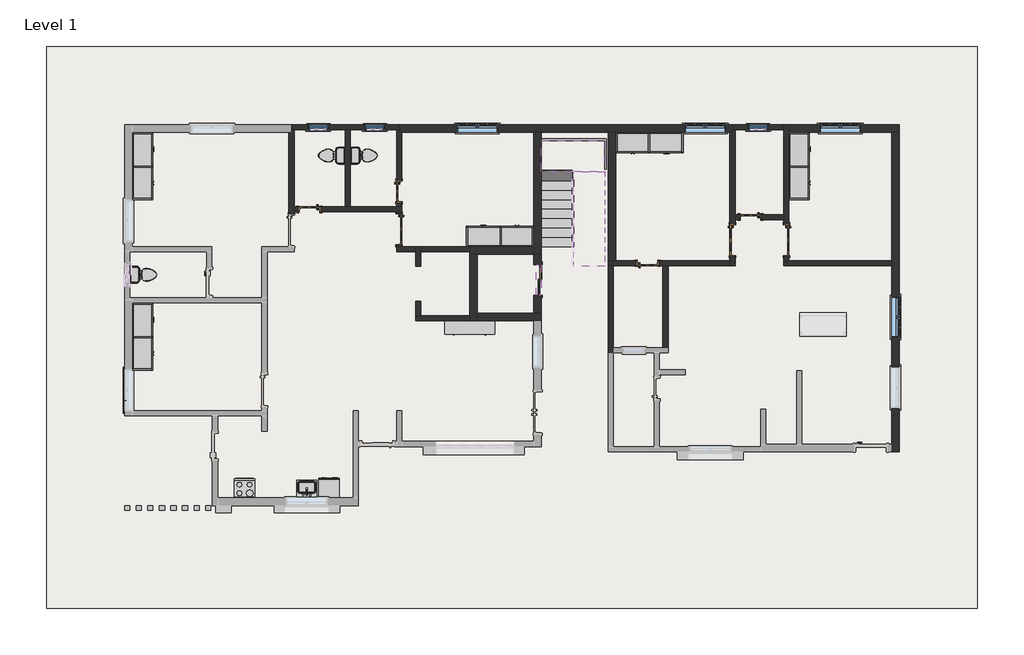
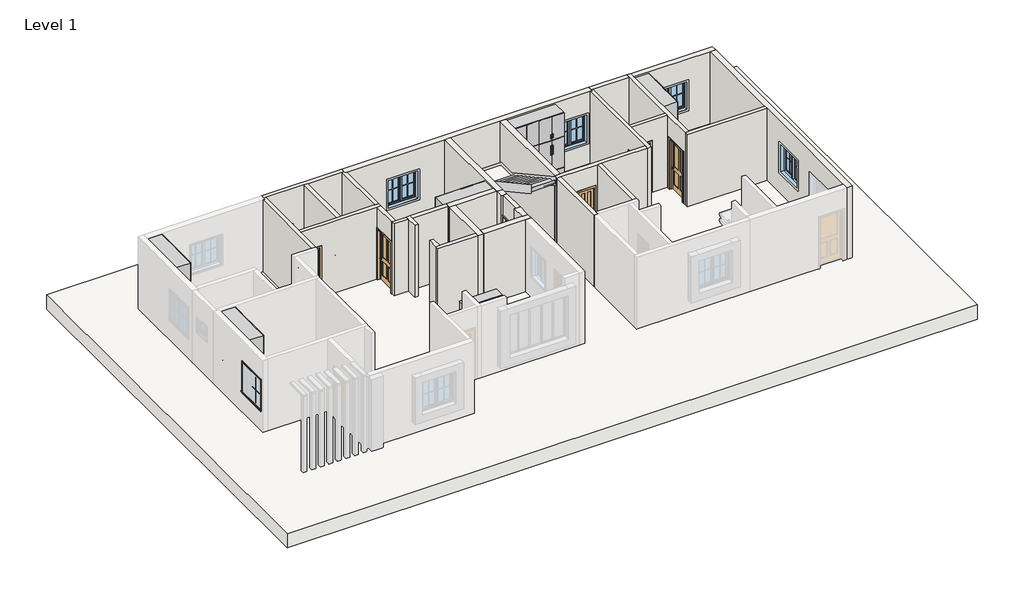
# One storey, part 2 of 3: 30 walls, 8 doors, 7 windows, 6 furniture elements, 4 flow terminals, 4 proxies, 2 slabs, 2 stair flights.
"""IFC4 building model written with IfcOpenShell, lengths in millimetres."""

from ifc_helpers import new_model, si_unit, frame, origin, origin_with_axes, place, context, project, spatial, polyline, outline, extrude, faceted_brep, transform, mapped, element, save
from components import dishwasher_m_610_x_610_x_860mm_47db8dec, muntin_pattern_2x2_muntin_pattern_2x2_4dfeb3f3, range_m_610_x_610mm_88bdc8d1, trim_window_exterior_flat_with_sill_7cfdd449, door_double_sliding_lift_3_x_7_7d4312a2, door_interior_single_4_panel_wood_2_x_7_0d1fc69e, door_interior_single_4_panel_wood_bed_door_3_x_7_ecef8289, door_interior_single_4_panel_wood_bed_door_3_x_7_5a83478c, m_sink_kitchen_single_760_x_535mm_2_83ebd6f4, toilet_domestic_3d_toilet_domestic_3d_ba6479b0, toilet_domestic_3d_toilet_domestic_3d_30431060, furniture_1wardrobe_6271_1wardrobe_6271_4dd35231, tv_stand_17254_tv_stand_17254_2bb553a4, non_monolithic_landing_f80fbcea, stair_flight_7b1ec15d, stair_flight_b2a94bac, window_casement_double_4_x_4_9200f5ac, window_double_hung_2_x_2_0206a36d

model = new_model("IFC4")

# Units and contexts
model_context = context("Model", 3, world=origin())
ifc_project = project(units=[si_unit("LENGTHUNIT", "METRE", prefix="MILLI")], contexts=[model_context])

# Site, building, storey
site = spatial("IfcSite", under=ifc_project)
building = spatial("IfcBuilding", under=site)
storey = spatial("IfcBuildingStorey", under=building, Name="Level 1", Elevation=0.0)

# Proxies
placement = place(None, origin())
dishwasher_m_610_x_610_x_860mm_shape = dishwasher_m_610_x_610_x_860mm_47db8dec(model_context)
element("IfcBuildingElementProxy", 1, Name="Dishwasher (M) : 610 x 610 x 860mm", ObjectType="Dishwasher (M) : 610 x 610 x 860mm", at=placement, inside=storey, context=model_context, shape_type="MappedRepresentation", body=[
    mapped(dishwasher_m_610_x_610_x_860mm_shape, transform((-5652.0362121, -4709.5777454, 0.0), x_axis=(-1.0, 0.0, 0.0), y_axis=(0.0, -1.0, 0.0), z_axis=(0.0, 0.0, 1.0))),
])
muntin_pattern_2x2_muntin_pattern_2x2_shape = muntin_pattern_2x2_muntin_pattern_2x2_4dfeb3f3(model_context)
element("IfcBuildingElementProxy", 2, Name="Muntin Pattern_2x2 : Muntin Pattern_2x2", ObjectType="Muntin Pattern_2x2 : Muntin Pattern_2x2", at=placement, inside=storey, context=model_context, shape_type="MappedRepresentation", body=[
    mapped(muntin_pattern_2x2_muntin_pattern_2x2_shape, transform((-12090.6286806, -2345.9398102, 984.25), x_axis=(0.0, 1.0, 0.0), y_axis=(-1.0, 0.0, 0.0), z_axis=(0.0, 0.0, 1.0))),
])
range_m_610_x_610mm_shape = range_m_610_x_610mm_88bdc8d1(model_context)
element("IfcBuildingElementProxy", 3, Name="Range (M) : 610 x 610mm", ObjectType="Range (M) : 610 x 610mm", at=placement, inside=storey, context=model_context, shape_type="MappedRepresentation", body=[
    mapped(range_m_610_x_610mm_shape, transform((-8237.1536806, -4671.2273102, 0.0), x_axis=(-1.0, 0.0, 0.0), y_axis=(0.0, -1.0, 0.0), z_axis=(0.0, 0.0, 1.0))),
])
trim_window_exterior_flat_with_sill_shape = trim_window_exterior_flat_with_sill_7cfdd449(model_context)
element("IfcBuildingElementProxy", 4, Name="Trim-Window-Exterior-Flat : with Sill", ObjectType="Trim-Window-Exterior-Flat : with Sill", at=placement, inside=storey, context=model_context, shape_type="MappedRepresentation", body=[
    mapped(trim_window_exterior_flat_with_sill_shape, transform((-12100.1536806, -2042.7273102, 2133.6), x_axis=(0.0, -1.0, 0.0), y_axis=(0.0, 0.0, 1.0), z_axis=(-1.0, 0.0, 0.0))),
])

# Doors
door_double_sliding_lift_3_x_7_shape = door_double_sliding_lift_3_x_7_7d4312a2(model_context)
element("IfcDoor", 5, ObjectType="Door-Double-Sliding : LIFT 3' X 7'", at=placement, inside=storey, context=model_context, shape_type="MappedRepresentation", body=[
    mapped(door_double_sliding_lift_3_x_7_shape, transform((79.1463194, 1233.8726898, 0.0), x_axis=(0.0, -1.0, 0.0), y_axis=(1.0, 0.0, 0.0), z_axis=(0.0, 0.0, 1.0))),
])
door_interior_single_4_panel_wood_2_x_7_shape = door_interior_single_4_panel_wood_2_x_7_0d1fc69e(model_context)
element("IfcDoor", 6, ObjectType="Door-Interior-Single-4_Panel-Wood : 2' X 7'", at=placement, inside=storey, context=model_context, shape_type="MappedRepresentation", body=[
    mapped(door_interior_single_4_panel_wood_2_x_7_shape, transform((-6613.7536806, 3332.5476898, 0.0), x_axis=(-1.0, 0.0, 0.0), y_axis=(0.0, -1.0, 0.0), z_axis=(0.0, 0.0, 1.0))),
])
element("IfcDoor", 7, ObjectType="Door-Interior-Single-4_Panel-Wood : 2' X 7'", at=placement, inside=storey, context=model_context, shape_type="MappedRepresentation", body=[
    mapped(door_interior_single_4_panel_wood_2_x_7_shape, transform((-3949.9286806, 3862.7726898, 0.0), x_axis=(0.0, -1.0, 0.0), y_axis=(1.0, 0.0, 0.0), z_axis=(0.0, 0.0, 1.0))),
])
element("IfcDoor", 8, ObjectType="Door-Interior-Single-4_Panel-Wood : 2' X 7'", at=placement, inside=storey, context=model_context, shape_type="MappedRepresentation", body=[
    mapped(door_interior_single_4_panel_wood_2_x_7_shape, transform((3431.9463194, 1725.9976898, 0.0), x_axis=(1.0, 0.0, 0.0), y_axis=(0.0, 1.0, 0.0), z_axis=(0.0, 0.0, 1.0))),
])
element("IfcDoor", 9, ObjectType="Door-Interior-Single-4_Panel-Wood : 2' X 7'", at=placement, inside=storey, context=model_context, shape_type="MappedRepresentation", body=[
    mapped(door_interior_single_4_panel_wood_2_x_7_shape, transform((6492.6463194, 3103.9476898, 0.0), x_axis=(-1.0, 0.0, 0.0), y_axis=(0.0, -1.0, 0.0), z_axis=(0.0, 0.0, 1.0))),
])
door_interior_single_4_panel_wood_bed_door_3_x_7_shape = door_interior_single_4_panel_wood_bed_door_3_x_7_ecef8289(model_context)
element("IfcDoor", 10, ObjectType="Door-Interior-Single-4_Panel-Wood : BED DOOR 3' X 7'", at=placement, inside=storey, context=model_context, shape_type="MappedRepresentation", body=[
    mapped(door_interior_single_4_panel_wood_bed_door_3_x_7_shape, transform((7562.6213194, 2414.9726898, 0.0), x_axis=(0.0, -1.0, 0.0), y_axis=(1.0, 0.0, 0.0), z_axis=(0.0, 0.0, 1.0))),
])
element("IfcDoor", 11, ObjectType="Door-Interior-Single-4_Panel-Wood : BED DOOR 3' X 7'", at=placement, inside=storey, context=model_context, shape_type="MappedRepresentation", body=[
    mapped(door_interior_single_4_panel_wood_bed_door_3_x_7_shape, transform((-3943.4688082, 2738.7747509, 0.0), x_axis=(0.0, -1.0, 0.0), y_axis=(1.0, 0.0, 0.0), z_axis=(0.0, 0.0, 1.0))),
])
door_interior_single_4_panel_wood_bed_door_3_x_7_2_shape = door_interior_single_4_panel_wood_bed_door_3_x_7_5a83478c(model_context)
element("IfcDoor", 12, ObjectType="Door-Interior-Single-4_Panel-Wood : BED DOOR 3' X 7'", at=placement, inside=storey, context=model_context, shape_type="MappedRepresentation", body=[
    mapped(door_interior_single_4_panel_wood_bed_door_3_x_7_2_shape, transform((5956.0713194, 2414.9726898, 0.0), x_axis=(0.0, -1.0, 0.0), y_axis=(1.0, 0.0, 0.0), z_axis=(0.0, 0.0, 1.0))),
])

# Flow terminals
m_sink_kitchen_single_760_x_535mm_2_shape = m_sink_kitchen_single_760_x_535mm_2_83ebd6f4(model_context)
element("IfcFlowTerminal", 13, ObjectType="M_Sink Kitchen-Single : 760 x 535mm 2", at=placement, inside=storey, context=model_context, shape_type="MappedRepresentation", body=[
    mapped(m_sink_kitchen_single_760_x_535mm_2_shape, transform((-6707.8429211, -4961.181909, 0.0), x_axis=(1.0, 0.0, 0.0), y_axis=(0.0, 1.0, 0.0), z_axis=(0.0, 0.0, 1.0))),
])
toilet_domestic_3d_toilet_domestic_3d_shape = toilet_domestic_3d_toilet_domestic_3d_ba6479b0(model_context)
toilet_domestic_3d_toilet_domestic_3d_2_shape = toilet_domestic_3d_toilet_domestic_3d_30431060(model_context)
element("IfcFlowTerminal", 14, ObjectType="Toilet-Domestic-3D : Toilet-Domestic-3D", at=placement, inside=storey, context=model_context, shape_type="MappedRepresentation", body=[
    mapped(toilet_domestic_3d_toilet_domestic_3d_shape, transform((-11453.0576532, 1386.2726898, 0.0), x_axis=(0.0, 1.0, 0.0), y_axis=(-1.0, 0.0, 0.0), z_axis=(0.0, 0.0, 1.0))),
    mapped(toilet_domestic_3d_toilet_domestic_3d_2_shape, transform((-11453.0576532, 1386.2726898, 0.0), x_axis=(0.0, 1.0, 0.0), y_axis=(-1.0, 0.0, 0.0), z_axis=(0.0, 0.0, 1.0))),
])
element("IfcFlowTerminal", 15, ObjectType="Toilet-Domestic-3D : Toilet-Domestic-3D", at=placement, inside=storey, context=model_context, shape_type="MappedRepresentation", body=[
    mapped(toilet_domestic_3d_toilet_domestic_3d_shape, transform((-6041.6497079, 4929.5726898, 0.0), x_axis=(0.0, -1.0, 0.0), y_axis=(1.0, 0.0, 0.0), z_axis=(0.0, 0.0, 1.0))),
    mapped(toilet_domestic_3d_toilet_domestic_3d_2_shape, transform((-6041.6497079, 4929.5726898, 0.0), x_axis=(0.0, -1.0, 0.0), y_axis=(1.0, 0.0, 0.0), z_axis=(0.0, 0.0, 1.0))),
])
element("IfcFlowTerminal", 16, ObjectType="Toilet-Domestic-3D : Toilet-Domestic-3D", at=placement, inside=storey, context=model_context, shape_type="MappedRepresentation", body=[
    mapped(toilet_domestic_3d_toilet_domestic_3d_shape, transform((-4899.8576532, 4929.5726898, 0.0), x_axis=(0.0, 1.0, 0.0), y_axis=(-1.0, 0.0, 0.0), z_axis=(0.0, 0.0, 1.0))),
    mapped(toilet_domestic_3d_toilet_domestic_3d_2_shape, transform((-4899.8576532, 4929.5726898, 0.0), x_axis=(0.0, 1.0, 0.0), y_axis=(-1.0, 0.0, 0.0), z_axis=(0.0, 0.0, 1.0))),
])

# Furniture
furniture_1wardrobe_6271_1wardrobe_6271_shape = furniture_1wardrobe_6271_1wardrobe_6271_4dd35231(model_context)
element("IfcFurniture", 17, ObjectType="1Wardrobe_6271 : 1Wardrobe_6271", at=placement, inside=storey, context=model_context, shape_type="MappedRepresentation", body=[
    mapped(furniture_1wardrobe_6271_1wardrobe_6271_shape, transform((-11871.5536806, 3615.3726898, 0.0), x_axis=(0.0, 1.0, 0.0), y_axis=(-1.0, 0.0, 0.0), z_axis=(0.0, 0.0, 1.0))),
])
element("IfcFurniture", 18, ObjectType="1Wardrobe_6271 : 1Wardrobe_6271", at=placement, inside=storey, context=model_context, shape_type="MappedRepresentation", body=[
    mapped(furniture_1wardrobe_6271_1wardrobe_6271_shape, transform((2492.1463194, 5615.3726898, 0.0), x_axis=(1.0, 0.0, 0.0), y_axis=(0.0, 1.0, 0.0), z_axis=(0.0, 0.0, 1.0))),
])
element("IfcFurniture", 19, ObjectType="1Wardrobe_6271 : 1Wardrobe_6271", at=placement, inside=storey, context=model_context, shape_type="MappedRepresentation", body=[
    mapped(furniture_1wardrobe_6271_1wardrobe_6271_shape, transform((7635.6463194, 3615.3726898, 0.0), x_axis=(0.0, 1.0, 0.0), y_axis=(-1.0, 0.0, 0.0), z_axis=(0.0, 0.0, 1.0))),
])
element("IfcFurniture", 20, ObjectType="1Wardrobe_6271 : 1Wardrobe_6271", at=placement, inside=storey, context=model_context, shape_type="MappedRepresentation", body=[
    mapped(furniture_1wardrobe_6271_1wardrobe_6271_shape, transform((-11871.5536806, -1451.9273102, 0.0), x_axis=(0.0, 1.0, 0.0), y_axis=(-1.0, 0.0, 0.0), z_axis=(0.0, 0.0, 1.0))),
])
element("IfcFurniture", 21, ObjectType="1Wardrobe_6271 : 1Wardrobe_6271", at=placement, inside=storey, context=model_context, shape_type="MappedRepresentation", body=[
    mapped(furniture_1wardrobe_6271_1wardrobe_6271_shape, transform((53.7463194, 2224.4726898, 0.0), x_axis=(-1.0, 0.0, 0.0), y_axis=(0.0, -1.0, 0.0), z_axis=(0.0, 0.0, 1.0))),
])
tv_stand_17254_tv_stand_17254_shape = tv_stand_17254_tv_stand_17254_2bb553a4(model_context)
element("IfcFurniture", 22, ObjectType="TV_Stand_17254 : TV_Stand_17254", at=placement, inside=storey, context=model_context, shape_type="MappedRepresentation", body=[
    mapped(tv_stand_17254_tv_stand_17254_shape, transform((-1851.2536806, 14.6726898, 0.0), x_axis=(-1.0, 0.0, 0.0), y_axis=(0.0, -1.0, 0.0), z_axis=(0.0, 0.0, 1.0))),
])

# Slabs
element("IfcSlab", 23, ObjectType="2'", at=placement, inside=storey, context=model_context, shape_type="SweptSolid", body=[
    extrude(outline(polyline([(13236.3463194, 8168.0726898), (13236.3463194, -8519.7273102), (-14424.2536806, -8519.7273102), (-14424.2536806, 8168.0726898), (13236.3463194, 8168.0726898)])), frame((0.0, 0.0, -609.6), z_axis=(0.0, 0.0, 1.0), x_axis=(1.0, 0.0, 0.0)), (0.0, 0.0, 1.0), 609.6),
])
non_monolithic_landing_shape = non_monolithic_landing_f80fbcea(model_context)
element("IfcSlab", 24, ObjectType="Non-Monolithic Landing", at=placement, inside=storey, context=model_context, shape_type="MappedRepresentation", body=[
    mapped(non_monolithic_landing_shape, transform((0.0, 0.0, 0.0), x_axis=(1.0, 0.0, 0.0), y_axis=(0.0, 1.0, 0.0), z_axis=(0.0, 0.0, 1.0))),
])

# Stair flights
stair_flight_shape = stair_flight_7b1ec15d(model_context)
element("IfcStairFlight", 25, ObjectType="2\" Tread 1\" Nosing 1/4\" Riser", at=placement, inside=storey, context=model_context, shape_type="MappedRepresentation", body=[
    mapped(stair_flight_shape, transform((0.0, 0.0, 0.0), x_axis=(1.0, 0.0, 0.0), y_axis=(0.0, 1.0, 0.0), z_axis=(0.0, 0.0, 1.0))),
])
stair_flight_2_shape = stair_flight_b2a94bac(model_context)
element("IfcStairFlight", 26, ObjectType="2\" Tread 1\" Nosing 1/4\" Riser", at=placement, inside=storey, context=model_context, shape_type="MappedRepresentation", body=[
    mapped(stair_flight_2_shape, transform((0.0, 0.0, 0.0), x_axis=(1.0, 0.0, 0.0), y_axis=(0.0, 1.0, 0.0), z_axis=(0.0, 0.0, 1.0))),
])

# Walls
element("IfcWall", 27, ObjectType="6\"", at=placement, inside=storey, context=model_context, shape_type="Brep", body=[
    faceted_brep([(-7147.1536806, 5691.5726898, 0.0), (-7070.9536806, 5691.5726898, 0.0), (-5546.9536806, 5691.5726898, 0.0), (-5394.5536806, 5691.5726898, 0.0), (-4022.9536806, 5691.5726898, 0.0), (-3946.7536806, 5691.5726898, 0.0), (-3946.7536806, 5691.5726898, 3048.0), (-4022.9536806, 5691.5726898, 3048.0), (-5394.5536806, 5691.5726898, 3048.0), (-5546.9536806, 5691.5726898, 3048.0), (-7070.9536806, 5691.5726898, 3048.0), (-7147.1536806, 5691.5726898, 3048.0), (-6042.2536806, 5691.5726898, 1511.3), (-6042.2536806, 5691.5726898, 914.4), (-6651.8536806, 5691.5726898, 914.4), (-6651.8536806, 5691.5726898, 1511.3), (-4365.8536806, 5691.5726898, 1511.3), (-4365.8536806, 5691.5726898, 914.4), (-4975.4536806, 5691.5726898, 914.4), (-4975.4536806, 5691.5726898, 1511.3), (-7147.1536806, 5843.9726898, 0.0), (-7147.1536806, 5843.9726898, 3048.0), (-3946.7536806, 5843.9726898, 3048.0), (-3946.7536806, 5843.9726898, 0.0), (-6042.2536806, 5843.9726898, 1511.3), (-6651.8536806, 5843.9726898, 1511.3), (-6651.8536806, 5843.9726898, 914.4), (-6042.2536806, 5843.9726898, 914.4), (-4365.8536806, 5843.9726898, 1511.3), (-4975.4536806, 5843.9726898, 1511.3), (-4975.4536806, 5843.9726898, 914.4), (-4365.8536806, 5843.9726898, 914.4)], [[[0, 1, 2, 3, 4, 5, 6, 7, 8, 9, 10, 11], [12, 13, 14, 15], [16, 17, 18, 19]], [[20, 21, 22, 23], [24, 25, 26, 27], [28, 29, 30, 31]], [[5, 4, 3, 2, 1, 0, 20, 23]], [[6, 5, 23, 22]], [[11, 10, 9, 8, 7, 6, 22, 21]], [[0, 11, 21, 20]], [[13, 12, 24, 27]], [[14, 13, 27, 26]], [[15, 14, 26, 25]], [[12, 15, 25, 24]], [[17, 16, 28, 31]], [[18, 17, 31, 30]], [[19, 18, 30, 29]], [[16, 19, 29, 28]]]),
])
element("IfcWall", 28, ObjectType="6\"", at=placement, inside=storey, context=model_context, shape_type="Brep", body=[
    faceted_brep([(-7070.9536806, 5691.5726898, 3048.0), (-7070.9536806, 3405.5726898, 3048.0), (-7070.9536806, 3253.1726898, 3048.0), (-7070.9536806, 2224.4726898, 3048.0), (-7070.9536806, 2224.4726898, 2159.0), (-7070.9536806, 3183.3226898, 2159.0), (-7070.9536806, 3183.3226898, 0.0), (-7070.9536806, 3253.1726898, 0.0), (-7070.9536806, 3405.5726898, 0.0), (-7070.9536806, 5691.5726898, 0.0), (-7223.3536806, 5615.3726898, 3048.0), (-7223.3536806, 5615.3726898, 0.0), (-7223.3536806, 3183.3226898, 0.0), (-7223.3536806, 3183.3226898, 2159.0), (-7223.3536806, 2224.4726898, 2159.0), (-7223.3536806, 2224.4726898, 3048.0), (-7147.1536806, 5615.3726898, 0.0), (-7147.1536806, 5691.5726898, 0.0), (-7147.1536806, 5691.5726898, 3048.0), (-7147.1536806, 5615.3726898, 3048.0)], [[[0, 1, 2, 3, 4, 5, 6, 7, 8, 9]], [[10, 11, 12, 13, 14, 15]], [[11, 16, 17, 9, 8, 7, 6, 12]], [[3, 2, 1, 0, 18, 19, 10, 15]], [[3, 15, 14, 4]], [[0, 9, 17, 18]], [[17, 16, 19, 18]], [[11, 10, 19, 16]], [[13, 5, 4, 14]], [[5, 13, 12, 6]]]),
])
element("IfcWall", 29, ObjectType="6\"", at=placement, inside=storey, context=model_context, shape_type="Brep", body=[
    faceted_brep([(-3870.5536806, 3253.1726898, 3048.0), (-4022.8438082, 3253.1726898, 3048.0), (-7070.9536806, 3253.1726898, 3048.0), (-7070.9536806, 3253.1726898, 0.0), (-6943.9536806, 3253.1726898, 0.0), (-6943.9536806, 3253.1726898, 2159.0), (-6283.5536806, 3253.1726898, 2159.0), (-6283.5536806, 3253.1726898, 0.0), (-4022.8438082, 3253.1726898, 0.0), (-3870.5536806, 3253.1726898, 0.0), (-7070.9536806, 3405.5726898, 3048.0), (-5546.9536806, 3405.5726898, 3048.0), (-5394.5536806, 3405.5726898, 3048.0), (-4022.9536806, 3405.5726898, 3048.0), (-3870.5536806, 3405.5726898, 3048.0), (-3870.5536806, 3405.5726898, 0.0), (-4022.9536806, 3405.5726898, 0.0), (-5394.5536806, 3405.5726898, 0.0), (-5546.9536806, 3405.5726898, 0.0), (-6283.5536806, 3405.5726898, 0.0), (-6283.5536806, 3405.5726898, 2159.0), (-6943.9536806, 3405.5726898, 2159.0), (-6943.9536806, 3405.5726898, 0.0), (-7070.9536806, 3405.5726898, 0.0)], [[[0, 1, 2, 3, 4, 5, 6, 7, 8, 9]], [[10, 11, 12, 13, 14, 15, 16, 17, 18, 19, 20, 21, 22, 23]], [[3, 23, 22, 4]], [[15, 9, 8, 7, 19, 18, 17, 16]], [[2, 1, 0, 14, 13, 12, 11, 10]], [[3, 2, 10, 23]], [[0, 9, 15, 14]], [[21, 5, 4, 22]], [[5, 21, 20, 6]], [[6, 20, 19, 7]]]),
])
element("IfcWall", 30, ObjectType="6\"", at=placement, inside=storey, context=model_context, shape_type="SweptSolid", body=[
    extrude(outline(polyline([(-5394.5536806, 5691.5726898), (-5394.5536806, 3405.5726898), (-5546.9536806, 3405.5726898), (-5546.9536806, 5691.5726898), (-5394.5536806, 5691.5726898)])), origin_with_axes(), (0.0, 0.0, 1.0), 3048.0),
])
element("IfcWall", 31, ObjectType="6\"", at=placement, inside=storey, context=model_context, shape_type="Brep", body=[
    faceted_brep([(-3870.5536806, 5615.3726898, 3048.0), (-3870.5536806, 3405.5726898, 3048.0), (-3870.5536806, 3405.5726898, 0.0), (-3870.5536806, 3532.5726898, 0.0), (-3870.5536806, 3532.5726898, 2159.0), (-3870.5536806, 4192.9726898, 2159.0), (-3870.5536806, 4192.9726898, 0.0), (-3870.5536806, 5615.3726898, 0.0), (-4022.9536806, 5691.5726898, 3048.0), (-4022.9536806, 5691.5726898, 0.0), (-4022.9536806, 4192.9726898, 0.0), (-4022.9536806, 4192.9726898, 2159.0), (-4022.9536806, 3532.5726898, 2159.0), (-4022.9536806, 3532.5726898, 0.0), (-4022.9536806, 3405.5726898, 0.0), (-4022.9536806, 3405.5726898, 3048.0), (-3946.7536806, 5691.5726898, 0.0), (-3946.7536806, 5615.3726898, 0.0), (-3946.7536806, 5615.3726898, 3048.0), (-3946.7536806, 5691.5726898, 3048.0)], [[[0, 1, 2, 3, 4, 5, 6, 7]], [[8, 9, 10, 11, 12, 13, 14, 15]], [[2, 14, 13, 3]], [[9, 16, 17, 7, 6, 10]], [[1, 0, 18, 19, 8, 15]], [[2, 1, 15, 14]], [[0, 7, 17, 18]], [[17, 16, 19, 18]], [[9, 8, 19, 16]], [[12, 4, 3, 13]], [[4, 12, 11, 5]], [[5, 11, 10, 6]]]),
])
element("IfcWall", 32, ObjectType="6\"", at=placement, inside=storey, context=model_context, shape_type="Brep", body=[
    faceted_brep([(2263.5463194, 1652.9726898, 0.0), (2263.5463194, -937.8273102, 0.0), (2263.5463194, -937.8273102, 3048.0), (2263.5463194, 1652.9726898, 3048.0), (2415.9463194, 1652.9726898, 0.0), (2415.9463194, 1652.9726898, 3048.0), (2415.9463194, -785.4273102, 3048.0), (2415.9463194, -937.8273102, 3048.0), (2415.9463194, -937.8273102, 0.0), (2415.9463194, -785.4273102, 0.0)], [[[0, 1, 2, 3]], [[4, 5, 6, 7, 8, 9]], [[1, 0, 4, 9, 8]], [[3, 2, 7, 6, 5]], [[2, 1, 8, 7]], [[0, 3, 5, 4]]]),
])
element("IfcWall", 33, ObjectType="6\"", at=placement, inside=storey, context=model_context, shape_type="Brep", body=[
    faceted_brep([(5883.0463194, 1652.9726898, 3048.0), (5883.0463194, 1805.3726898, 3048.0), (5883.0463194, 5615.3726898, 3048.0), (5883.0463194, 5615.3726898, 0.0), (5883.0463194, 2897.5726898, 0.0), (5883.0463194, 2897.5726898, 2159.0), (5883.0463194, 1932.3726898, 2159.0), (5883.0463194, 1932.3726898, 0.0), (5883.0463194, 1805.3726898, 0.0), (5883.0463194, 1652.9726898, 0.0), (6035.4463194, 5691.5726898, 3048.0), (6035.4463194, 3176.9726898, 3048.0), (6035.4463194, 3024.5726898, 3048.0), (6035.4463194, 1652.9726898, 3048.0), (6035.4463194, 1652.9726898, 0.0), (6035.4463194, 1932.3726898, 0.0), (6035.4463194, 1932.3726898, 2159.0), (6035.4463194, 2897.5726898, 2159.0), (6035.4463194, 2897.5726898, 0.0), (6035.4463194, 3024.5726898, 0.0), (6035.4463194, 3176.9726898, 0.0), (6035.4463194, 5691.5726898, 0.0), (5959.2463194, 5615.3726898, 0.0), (5959.2463194, 5691.5726898, 0.0), (5959.2463194, 5691.5726898, 3048.0), (5959.2463194, 5615.3726898, 3048.0)], [[[0, 1, 2, 3, 4, 5, 6, 7, 8, 9]], [[10, 11, 12, 13, 14, 15, 16, 17, 18, 19, 20, 21]], [[14, 9, 8, 7, 15]], [[3, 22, 23, 21, 20, 19, 18, 4]], [[2, 1, 0, 13, 12, 11, 10, 24, 25]], [[0, 9, 14, 13]], [[3, 2, 25, 22]], [[25, 24, 23, 22]], [[10, 21, 23, 24]], [[6, 16, 15, 7]], [[16, 6, 5, 17]], [[17, 5, 4, 18]]]),
])
element("IfcWall", 34, ObjectType="6\"", at=placement, inside=storey, context=model_context, shape_type="Brep", body=[
    faceted_brep([(2263.5463194, 1805.3726898, 3048.0), (2492.1463194, 1805.3726898, 3048.0), (5883.0463194, 1805.3726898, 3048.0), (5883.0463194, 1805.3726898, 0.0), (3762.1463194, 1805.3726898, 0.0), (3762.1463194, 1805.3726898, 2159.0), (3101.7463194, 1805.3726898, 2159.0), (3101.7463194, 1805.3726898, 0.0), (2492.1463194, 1805.3726898, 0.0), (2263.5463194, 1805.3726898, 0.0), (5883.0463194, 1652.9726898, 3048.0), (4041.5463194, 1652.9726898, 3048.0), (3889.1463194, 1652.9726898, 3048.0), (2415.9463194, 1652.9726898, 3048.0), (2263.5463194, 1652.9726898, 3048.0), (2263.5463194, 1652.9726898, 0.0), (2415.9463194, 1652.9726898, 0.0), (3101.7463194, 1652.9726898, 0.0), (3101.7463194, 1652.9726898, 2159.0), (3762.1463194, 1652.9726898, 2159.0), (3762.1463194, 1652.9726898, 0.0), (3889.1463194, 1652.9726898, 0.0), (4041.5463194, 1652.9726898, 0.0), (5883.0463194, 1652.9726898, 0.0)], [[[0, 1, 2, 3, 4, 5, 6, 7, 8, 9]], [[10, 11, 12, 13, 14, 15, 16, 17, 18, 19, 20, 21, 22, 23]], [[3, 23, 22, 21, 20, 4]], [[15, 9, 8, 7, 17, 16]], [[2, 1, 0, 14, 13, 12, 11, 10]], [[3, 2, 10, 23]], [[0, 9, 15, 14]], [[19, 5, 4, 20]], [[5, 19, 18, 6]], [[6, 18, 17, 7]]]),
])
element("IfcWall", 35, ObjectType="6\"", at=placement, inside=storey, context=model_context, shape_type="SweptSolid", body=[
    extrude(outline(polyline([(4041.5463194, 1652.9726898), (4041.5463194, -785.4273102), (3889.1463194, -785.4273102), (3889.1463194, 1652.9726898), (4041.5463194, 1652.9726898)])), origin_with_axes(), (0.0, 0.0, 1.0), 3048.0),
])
element("IfcWall", 36, ObjectType="6\"", at=placement, inside=storey, context=model_context, shape_type="Brep", body=[
    faceted_brep([(10683.6463194, 1805.3726898, 0.0), (7635.6463194, 1805.3726898, 0.0), (7483.2463194, 1805.3726898, 0.0), (7483.2463194, 1805.3726898, 3048.0), (7635.6463194, 1805.3726898, 3048.0), (10683.6463194, 1805.3726898, 3048.0), (10683.6463194, 1652.9726898, 0.0), (10683.6463194, 1652.9726898, 3048.0), (7483.2463194, 1652.9726898, 3048.0), (7483.2463194, 1652.9726898, 0.0)], [[[0, 1, 2, 3, 4, 5]], [[6, 7, 8, 9]], [[2, 1, 0, 6, 9]], [[5, 4, 3, 8, 7]], [[0, 5, 7, 6]], [[3, 2, 9, 8]]]),
])
element("IfcWall", 37, ObjectType="6\"", at=placement, inside=storey, context=model_context, shape_type="Brep", body=[
    faceted_brep([(7635.6463194, 5843.9726898, 3048.0), (7635.6463194, 5615.3726898, 3048.0), (7635.6463194, 1805.3726898, 3048.0), (7635.6463194, 1805.3726898, 0.0), (7635.6463194, 1932.3726898, 0.0), (7635.6463194, 1932.3726898, 2159.0), (7635.6463194, 2897.5726898, 2159.0), (7635.6463194, 2897.5726898, 0.0), (7635.6463194, 5615.3726898, 0.0), (7635.6463194, 5843.9726898, 0.0), (7483.2463194, 1805.3726898, 3048.0), (7483.2463194, 3024.5726898, 3048.0), (7483.2463194, 3176.9726898, 3048.0), (7483.2463194, 5691.5726898, 3048.0), (7483.2463194, 5843.9726898, 3048.0), (7483.2463194, 5843.9726898, 0.0), (7483.2463194, 5691.5726898, 0.0), (7483.2463194, 3176.9726898, 0.0), (7483.2463194, 3024.5726898, 0.0), (7483.2463194, 2897.5726898, 0.0), (7483.2463194, 2897.5726898, 2159.0), (7483.2463194, 1932.3726898, 2159.0), (7483.2463194, 1932.3726898, 0.0), (7483.2463194, 1805.3726898, 0.0)], [[[0, 1, 2, 3, 4, 5, 6, 7, 8, 9]], [[10, 11, 12, 13, 14, 15, 16, 17, 18, 19, 20, 21, 22, 23]], [[3, 23, 22, 4]], [[15, 9, 8, 7, 19, 18, 17, 16]], [[2, 1, 0, 14, 13, 12, 11, 10]], [[3, 2, 10, 23]], [[14, 0, 9, 15]], [[21, 5, 4, 22]], [[5, 21, 20, 6]], [[6, 20, 19, 7]]]),
])
element("IfcWall", 38, ObjectType="6\"", at=placement, inside=storey, context=model_context, shape_type="SweptSolid", body=[
    extrude(outline(polyline([(3048.0, 7483.2463194), (3048.0, 6035.4463194), (0.0, 6035.4463194), (0.0, 6162.4463194), (2159.0, 6162.4463194), (2159.0, 6822.8463194), (0.0, 6822.8463194), (0.0, 7483.2463194), (3048.0, 7483.2463194)])), frame((0.0, 3024.5726898, 0.0), z_axis=(0.0, 1.0, 0.0), x_axis=(0.0, 0.0, 1.0)), (0.0, 0.0, 1.0), 152.4),
])
element("IfcWall", 39, ObjectType="6\"", at=placement, inside=storey, context=model_context, shape_type="Brep", body=[
    faceted_brep([(5959.2463194, 5691.5726898, 0.0), (6035.4463194, 5691.5726898, 0.0), (7483.2463194, 5691.5726898, 0.0), (7483.2463194, 5691.5726898, 3048.0), (6035.4463194, 5691.5726898, 3048.0), (5959.2463194, 5691.5726898, 3048.0), (7026.0463194, 5691.5726898, 1511.3), (7026.0463194, 5691.5726898, 914.4), (6416.4463194, 5691.5726898, 914.4), (6416.4463194, 5691.5726898, 1511.3), (5959.2463194, 5843.9726898, 0.0), (5959.2463194, 5843.9726898, 3048.0), (7483.2463194, 5843.9726898, 3048.0), (7483.2463194, 5843.9726898, 0.0), (7026.0463194, 5843.9726898, 1511.3), (6416.4463194, 5843.9726898, 1511.3), (6416.4463194, 5843.9726898, 914.4), (7026.0463194, 5843.9726898, 914.4)], [[[0, 1, 2, 3, 4, 5], [6, 7, 8, 9]], [[10, 11, 12, 13], [14, 15, 16, 17]], [[2, 1, 0, 10, 13]], [[5, 4, 3, 12, 11]], [[0, 5, 11, 10]], [[3, 2, 13, 12]], [[7, 6, 14, 17]], [[8, 7, 17, 16]], [[9, 8, 16, 15]], [[6, 9, 15, 14]]]),
])
element("IfcWall", 40, ObjectType="6\"", at=placement, inside=storey, context=model_context, shape_type="SweptSolid", body=[
    extrude(outline(polyline([(129.9463194, 776.6726898), (129.9463194, 1691.0726898), (282.3463194, 1691.0726898), (282.3463194, 776.6726898), (129.9463194, 776.6726898)])), frame((0.0, 0.0, 2133.6), z_axis=(0.0, 0.0, 1.0), x_axis=(1.0, 0.0, 0.0)), (0.0, 0.0, 1.0), 914.4),
])
element("IfcWall", 41, ObjectType="6\"", at=placement, inside=storey, context=model_context, shape_type="Brep", body=[
    faceted_brep([(-1851.2536806, 167.0726898, 0.0), (-3299.0536806, 167.0726898, 0.0), (-3451.4536806, 167.0726898, 0.0), (-3451.4536806, 167.0726898, 3048.0), (-3299.0536806, 167.0726898, 3048.0), (-1851.2536806, 167.0726898, 3048.0), (-1851.2536806, 14.6726898, 0.0), (-1851.2536806, 14.6726898, 3048.0), (-3451.4536806, 14.6726898, 3048.0), (-3451.4536806, 14.6726898, 0.0)], [[[0, 1, 2, 3, 4, 5]], [[6, 7, 8, 9]], [[2, 1, 0, 6, 9]], [[5, 4, 3, 8, 7]], [[0, 5, 7, 6]], [[3, 2, 9, 8]]]),
])
element("IfcWall", 42, ObjectType="6\"", at=placement, inside=storey, context=model_context, shape_type="SweptSolid", body=[
    extrude(outline(polyline([(-3299.0536806, 598.8726898), (-3299.0536806, 167.0726898), (-3451.4536806, 167.0726898), (-3451.4536806, 598.8726898), (-3299.0536806, 598.8726898)])), origin_with_axes(), (0.0, 0.0, 1.0), 3048.0),
])
element("IfcWall", 43, ObjectType="6\"", at=placement, inside=storey, context=model_context, shape_type="SweptSolid", body=[
    extrude(outline(polyline([(-1851.2536806, 2071.976812), (-3299.0536806, 2071.976812), (-3299.0536806, 2224.376812), (-1851.2536806, 2224.376812), (-1851.2536806, 2071.976812)])), origin_with_axes(), (0.0, 0.0, 1.0), 3048.0),
])
element("IfcWall", 44, ObjectType="6\"", at=placement, inside=storey, context=model_context, shape_type="Brep", body=[
    faceted_brep([(-3299.0536806, 1640.176812, 0.0), (-3299.0536806, 2071.976812, 0.0), (-3299.0536806, 2224.376812, 0.0), (-3299.0536806, 2224.376812, 3048.0), (-3299.0536806, 2071.976812, 3048.0), (-3299.0536806, 1640.176812, 3048.0), (-3451.4536806, 1640.176812, 0.0), (-3451.4536806, 1640.176812, 3048.0), (-3451.4536806, 2071.976812, 3048.0), (-3451.4536806, 2224.376812, 3048.0), (-3451.4536806, 2224.376812, 0.0), (-3451.4536806, 2071.976812, 0.0)], [[[0, 1, 2, 3, 4, 5]], [[6, 7, 8, 9, 10, 11]], [[2, 1, 0, 6, 11, 10]], [[5, 4, 3, 9, 8, 7]], [[0, 5, 7, 6]], [[3, 2, 10, 9]]]),
])
element("IfcWall", 45, ObjectType="6\"", at=placement, inside=storey, context=model_context, shape_type="Brep", body=[
    faceted_brep([(-3451.4536806, 2224.376812, 0.0), (-3870.4438082, 2224.376812, 0.0), (-4022.8438082, 2224.376812, 0.0), (-4022.8438082, 2224.376812, 3048.0), (-3870.4438082, 2224.376812, 3048.0), (-3451.4536806, 2224.376812, 3048.0), (-3451.4536806, 2071.976812, 0.0), (-3451.4536806, 2071.976812, 3048.0), (-4022.8438082, 2071.976812, 3048.0), (-4022.8438082, 2071.976812, 0.0)], [[[0, 1, 2, 3, 4, 5]], [[6, 7, 8, 9]], [[2, 1, 0, 6, 9]], [[5, 4, 3, 8, 7]], [[0, 5, 7, 6]], [[3, 2, 9, 8]]]),
])
element("IfcWall", 46, ObjectType="6\"", at=placement, inside=storey, context=model_context, shape_type="SweptSolid", body=[
    extrude(outline(polyline([(2224.376812, 3048.0), (3253.1726898, 3048.0), (3253.1726898, 0.0), (3221.3747509, 0.0), (3221.3747509, 2159.0), (2256.1747509, 2159.0), (2256.1747509, 0.0), (2224.376812, 0.0), (2224.376812, 3048.0)])), frame((-4022.8438082, 0.0, 0.0), z_axis=(1.0, 0.0, 0.0), x_axis=(0.0, 1.0, 0.0)), (0.0, 0.0, 1.0), 152.4),
])
element("IfcWall", 47, ObjectType="9\"", at=placement, inside=storey, context=model_context, shape_type="Brep", body=[
    faceted_brep([(10683.6463194, 5615.3726898, 0.0), (10683.6463194, 1805.3726898, 0.0), (10683.6463194, 1652.9726898, 0.0), (10683.6463194, -3642.9273102, 0.0), (10683.6463194, -3871.5273102, 0.0), (10683.6463194, -3871.5273102, 3048.0), (10683.6463194, -3642.9273102, 3048.0), (10683.6463194, 1652.9726898, 3048.0), (10683.6463194, 1805.3726898, 3048.0), (10683.6463194, 5615.3726898, 3048.0), (10683.6463194, -480.6273102, 2133.6), (10683.6463194, -480.6273102, 914.4), (10683.6463194, 738.5726898, 914.4), (10683.6463194, 738.5726898, 2133.6), (10683.6463194, -2576.1273102, 2133.6), (10683.6463194, -2576.1273102, 914.4), (10683.6463194, -1356.9273102, 914.4), (10683.6463194, -1356.9273102, 2133.6), (10912.2463194, 5615.3726898, 0.0), (10912.2463194, 5615.3726898, 3048.0), (10912.2463194, -3871.5273102, 3048.0), (10912.2463194, -3871.5273102, 0.0), (10912.2463194, -480.6273102, 2133.6), (10912.2463194, 738.5726898, 2133.6), (10912.2463194, 738.5726898, 914.4), (10912.2463194, -480.6273102, 914.4), (10912.2463194, -2576.1273102, 2133.6), (10912.2463194, -1356.9273102, 2133.6), (10912.2463194, -1356.9273102, 914.4), (10912.2463194, -2576.1273102, 914.4)], [[[0, 1, 2, 3, 4, 5, 6, 7, 8, 9], [10, 11, 12, 13], [14, 15, 16, 17]], [[18, 19, 20, 21], [22, 23, 24, 25], [26, 27, 28, 29]], [[4, 3, 2, 1, 0, 18, 21]], [[5, 4, 21, 20]], [[9, 8, 7, 6, 5, 20, 19]], [[0, 9, 19, 18]], [[11, 10, 22, 25]], [[12, 11, 25, 24]], [[13, 12, 24, 23]], [[10, 13, 23, 22]], [[15, 14, 26, 29]], [[16, 15, 29, 28]], [[17, 16, 28, 27]], [[14, 17, 27, 26]]]),
])
element("IfcWall", 48, ObjectType="9\"", at=placement, inside=storey, context=model_context, shape_type="Brep", body=[
    faceted_brep([(-3946.7536806, 5615.3726898, 0.0), (-3870.5536806, 5615.3726898, 0.0), (53.7463194, 5615.3726898, 0.0), (282.3463194, 5615.3726898, 0.0), (2263.5463194, 5615.3726898, 0.0), (2492.1463194, 5615.3726898, 0.0), (5883.0463194, 5615.3726898, 0.0), (5959.2463194, 5615.3726898, 0.0), (5959.2463194, 5615.3726898, 3048.0), (5883.0463194, 5615.3726898, 3048.0), (2492.1463194, 5615.3726898, 3048.0), (2263.5463194, 5615.3726898, 3048.0), (282.3463194, 5615.3726898, 3048.0), (53.7463194, 5615.3726898, 3048.0), (-3870.5536806, 5615.3726898, 3048.0), (-3946.7536806, 5615.3726898, 3048.0), (-1013.0536806, 5615.3726898, 2133.6), (-1013.0536806, 5615.3726898, 914.4), (-2232.2536806, 5615.3726898, 914.4), (-2232.2536806, 5615.3726898, 2133.6), (5756.0463194, 5615.3726898, 2133.6), (5756.0463194, 5615.3726898, 914.4), (4536.8463194, 5615.3726898, 914.4), (4536.8463194, 5615.3726898, 2133.6), (-3946.7536806, 5843.9726898, 0.0), (-3946.7536806, 5843.9726898, 3048.0), (5959.2463194, 5843.9726898, 3048.0), (5959.2463194, 5843.9726898, 0.0), (-1013.0536806, 5843.9726898, 2133.6), (-2232.2536806, 5843.9726898, 2133.6), (-2232.2536806, 5843.9726898, 914.4), (-1013.0536806, 5843.9726898, 914.4), (5756.0463194, 5843.9726898, 2133.6), (4536.8463194, 5843.9726898, 2133.6), (4536.8463194, 5843.9726898, 914.4), (5756.0463194, 5843.9726898, 914.4), (-3946.7536806, 5691.5726898, 0.0), (5959.2463194, 5691.5726898, 0.0), (5959.2463194, 5691.5726898, 3048.0), (-3946.7536806, 5691.5726898, 3048.0)], [[[0, 1, 2, 3, 4, 5, 6, 7, 8, 9, 10, 11, 12, 13, 14, 15], [16, 17, 18, 19], [20, 21, 22, 23]], [[24, 25, 26, 27], [28, 29, 30, 31], [32, 33, 34, 35]], [[7, 6, 5, 4, 3, 2, 1, 0, 36, 24, 27, 37]], [[8, 7, 37, 27, 26, 38]], [[15, 14, 13, 12, 11, 10, 9, 8, 38, 26, 25, 39]], [[0, 15, 39, 25, 24, 36]], [[17, 16, 28, 31]], [[18, 17, 31, 30]], [[19, 18, 30, 29]], [[16, 19, 29, 28]], [[21, 20, 32, 35]], [[22, 21, 35, 34]], [[23, 22, 34, 33]], [[20, 23, 33, 32]]]),
])
element("IfcWall", 49, ObjectType="9\"", at=placement, inside=storey, context=model_context, shape_type="Brep", body=[
    faceted_brep([(53.7463194, 5615.3726898, 0.0), (53.7463194, 2224.4726898, 0.0), (53.7463194, 1995.8726898, 0.0), (53.7463194, 1995.8726898, 3048.0), (53.7463194, 2224.4726898, 3048.0), (53.7463194, 5615.3726898, 3048.0), (282.3463194, 5615.3726898, 0.0), (282.3463194, 5615.3726898, 3048.0), (282.3463194, 1995.8726898, 3048.0), (282.3463194, 1995.8726898, 0.0)], [[[0, 1, 2, 3, 4, 5]], [[6, 7, 8, 9]], [[2, 1, 0, 6, 9]], [[5, 4, 3, 8, 7]], [[0, 5, 7, 6]], [[3, 2, 9, 8]]]),
])
element("IfcWall", 50, ObjectType="9\"", at=placement, inside=storey, context=model_context, shape_type="Brep", body=[
    faceted_brep([(53.7463194, 2224.4726898, 0.0), (-1851.2536806, 2224.4726898, 0.0), (-1851.2536806, 2224.4726898, 3048.0), (53.7463194, 2224.4726898, 3048.0), (53.7463194, 1995.8726898, 0.0), (53.7463194, 1995.8726898, 3048.0), (-1622.6536806, 1995.8726898, 3048.0), (-1851.2536806, 1995.8726898, 3048.0), (-1851.2536806, 1995.8726898, 0.0), (-1622.6536806, 1995.8726898, 0.0), (-1851.2536806, 2071.976812, 0.0), (-1851.2536806, 2071.976812, 3048.0)], [[[0, 1, 2, 3]], [[4, 5, 6, 7, 8, 9]], [[1, 0, 4, 9, 8, 10]], [[3, 2, 11, 7, 6, 5]], [[0, 3, 5, 4]], [[2, 1, 10, 8, 7, 11]]]),
])
element("IfcWall", 51, ObjectType="9\"", at=placement, inside=storey, context=model_context, shape_type="Brep", body=[
    faceted_brep([(-1851.2536806, 1995.8726898, 0.0), (-1851.2536806, 167.0726898, 0.0), (-1851.2536806, 14.6726898, 0.0), (-1851.2536806, 14.6726898, 3048.0), (-1851.2536806, 167.0726898, 3048.0), (-1851.2536806, 1995.8726898, 3048.0), (-1622.6536806, 1995.8726898, 0.0), (-1622.6536806, 1995.8726898, 3048.0), (-1622.6536806, 243.2726898, 3048.0), (-1622.6536806, 14.6726898, 3048.0), (-1622.6536806, 14.6726898, 0.0), (-1622.6536806, 243.2726898, 0.0)], [[[0, 1, 2, 3, 4, 5]], [[6, 7, 8, 9, 10, 11]], [[2, 1, 0, 6, 11, 10]], [[5, 4, 3, 9, 8, 7]], [[0, 5, 7, 6]], [[3, 2, 10, 9]]]),
])
element("IfcWall", 52, ObjectType="9\"", at=placement, inside=storey, context=model_context, shape_type="Brep", body=[
    faceted_brep([(-1622.6536806, 14.6726898, 0.0), (53.7463194, 14.6726898, 0.0), (282.3463194, 14.6726898, 0.0), (282.3463194, 14.6726898, 3048.0), (53.7463194, 14.6726898, 3048.0), (-1622.6536806, 14.6726898, 3048.0), (-1622.6536806, 243.2726898, 0.0), (-1622.6536806, 243.2726898, 3048.0), (53.7463194, 243.2726898, 3048.0), (282.3463194, 243.2726898, 3048.0), (282.3463194, 243.2726898, 0.0), (53.7463194, 243.2726898, 0.0)], [[[0, 1, 2, 3, 4, 5]], [[6, 7, 8, 9, 10, 11]], [[2, 1, 0, 6, 11, 10]], [[5, 4, 3, 9, 8, 7]], [[0, 5, 7, 6]], [[3, 2, 10, 9]]]),
])
element("IfcWall", 53, ObjectType="9\"", at=placement, inside=storey, context=model_context, shape_type="Brep", body=[
    faceted_brep([(282.3463194, 243.2726898, 0.0), (282.3463194, 776.6726898, 0.0), (282.3463194, 776.6726898, 2133.6), (282.3463194, 776.6726898, 3048.0), (282.3463194, 243.2726898, 3048.0), (53.7463194, 243.2726898, 0.0), (53.7463194, 243.2726898, 3048.0), (53.7463194, 776.6726898, 3048.0), (53.7463194, 776.6726898, 0.0), (129.9463194, 776.6726898, 3048.0)], [[[0, 1, 2, 3, 4]], [[5, 6, 7, 8]], [[1, 0, 5, 8]], [[3, 2, 1, 8, 7, 9]], [[4, 3, 9, 7, 6]], [[0, 4, 6, 5]]]),
])
element("IfcWall", 54, ObjectType="9\"", at=placement, inside=storey, context=model_context, shape_type="SweptSolid", body=[
    extrude(outline(polyline([(2263.5463194, 1805.3726898), (2263.5463194, 5615.3726898), (2492.1463194, 5615.3726898), (2492.1463194, 1805.3726898), (2263.5463194, 1805.3726898)])), origin_with_axes(), (0.0, 0.0, 1.0), 3048.0),
])
element("IfcWall", 55, ObjectType="9\"", at=placement, inside=storey, context=model_context, shape_type="Brep", body=[
    faceted_brep([(7635.6463194, 5615.3726898, 0.0), (10683.6463194, 5615.3726898, 0.0), (10912.2463194, 5615.3726898, 0.0), (10912.2463194, 5615.3726898, 3048.0), (10683.6463194, 5615.3726898, 3048.0), (7635.6463194, 5615.3726898, 3048.0), (9769.2463194, 5615.3726898, 2133.6), (9769.2463194, 5615.3726898, 914.4), (8550.0463194, 5615.3726898, 914.4), (8550.0463194, 5615.3726898, 2133.6), (7635.6463194, 5843.9726898, 0.0), (7635.6463194, 5843.9726898, 3048.0), (10912.2463194, 5843.9726898, 3048.0), (10912.2463194, 5843.9726898, 0.0), (9769.2463194, 5843.9726898, 2133.6), (8550.0463194, 5843.9726898, 2133.6), (8550.0463194, 5843.9726898, 914.4), (9769.2463194, 5843.9726898, 914.4)], [[[0, 1, 2, 3, 4, 5], [6, 7, 8, 9]], [[10, 11, 12, 13], [14, 15, 16, 17]], [[2, 1, 0, 10, 13]], [[5, 4, 3, 12, 11]], [[3, 2, 13, 12]], [[0, 5, 11, 10]], [[7, 6, 14, 17]], [[8, 7, 17, 16]], [[9, 8, 16, 15]], [[6, 9, 15, 14]]]),
])
element("IfcWall", 56, ObjectType="9\"", at=placement, inside=storey, context=model_context, shape_type="Brep", body=[
    faceted_brep([(282.3463194, 1691.0726898, 0.0), (282.3463194, 1995.8726898, 0.0), (282.3463194, 1995.8726898, 3048.0), (282.3463194, 1691.0726898, 3048.0), (282.3463194, 1691.0726898, 2133.6), (53.7463194, 1691.0726898, 0.0), (53.7463194, 1691.0726898, 3048.0), (53.7463194, 1995.8726898, 3048.0), (53.7463194, 1995.8726898, 0.0), (129.9463194, 1691.0726898, 3048.0)], [[[0, 1, 2, 3, 4]], [[5, 6, 7, 8]], [[1, 0, 5, 8]], [[3, 2, 7, 6, 9]], [[0, 4, 3, 9, 6, 5]], [[2, 1, 8, 7]]]),
])

# Windows
window_casement_double_4_x_4_shape = window_casement_double_4_x_4_9200f5ac(model_context)
element("IfcWindow", 57, ObjectType="Window-Casement-Double : 4' X 4'", at=placement, inside=storey, context=model_context, shape_type="MappedRepresentation", body=[
    mapped(window_casement_double_4_x_4_shape, transform((-1622.6536806, 5729.6726898, 0.0), x_axis=(1.0, 0.0, 0.0), y_axis=(0.0, 1.0, 0.0), z_axis=(0.0, 0.0, 1.0))),
])
element("IfcWindow", 58, ObjectType="Window-Casement-Double : 4' X 4'", at=placement, inside=storey, context=model_context, shape_type="MappedRepresentation", body=[
    mapped(window_casement_double_4_x_4_shape, transform((5146.4463194, 5729.6726898, 0.0), x_axis=(1.0, 0.0, 0.0), y_axis=(0.0, 1.0, 0.0), z_axis=(0.0, 0.0, 1.0))),
])
element("IfcWindow", 59, ObjectType="Window-Casement-Double : 4' X 4'", at=placement, inside=storey, context=model_context, shape_type="MappedRepresentation", body=[
    mapped(window_casement_double_4_x_4_shape, transform((9159.6463194, 5729.6726898, 0.0), x_axis=(1.0, 0.0, 0.0), y_axis=(0.0, 1.0, 0.0), z_axis=(0.0, 0.0, 1.0))),
])
element("IfcWindow", 60, ObjectType="Window-Casement-Double : 4' X 4'", at=placement, inside=storey, context=model_context, shape_type="MappedRepresentation", body=[
    mapped(window_casement_double_4_x_4_shape, transform((10797.9463194, 128.9726898, 0.0), x_axis=(0.0, -1.0, 0.0), y_axis=(1.0, 0.0, 0.0), z_axis=(0.0, 0.0, 1.0))),
])
window_double_hung_2_x_2_shape = window_double_hung_2_x_2_0206a36d(model_context)
element("IfcWindow", 61, ObjectType="Window-Double-Hung : 2' X 2'", at=placement, inside=storey, context=model_context, shape_type="MappedRepresentation", body=[
    mapped(window_double_hung_2_x_2_shape, transform((-6347.0536806, 5767.7726898, 0.0), x_axis=(-1.0, 0.0, 0.0), y_axis=(0.0, -1.0, 0.0), z_axis=(0.0, 0.0, 1.0))),
])
element("IfcWindow", 62, ObjectType="Window-Double-Hung : 2' X 2'", at=placement, inside=storey, context=model_context, shape_type="MappedRepresentation", body=[
    mapped(window_double_hung_2_x_2_shape, transform((-4670.6536806, 5767.7726898, 0.0), x_axis=(-1.0, 0.0, 0.0), y_axis=(0.0, -1.0, 0.0), z_axis=(0.0, 0.0, 1.0))),
])
element("IfcWindow", 63, ObjectType="Window-Double-Hung : 2' X 2'", at=placement, inside=storey, context=model_context, shape_type="MappedRepresentation", body=[
    mapped(window_double_hung_2_x_2_shape, transform((6721.2463194, 5767.7726898, 0.0), x_axis=(-1.0, 0.0, 0.0), y_axis=(0.0, -1.0, 0.0), z_axis=(0.0, 0.0, 1.0))),
])

save(model, "model.ifc")

# Revit data of these elements
# Type "Dishwasher (M) : 610 x 610 x 860mm"
#   Label = "DW"
#   Depth = 2' - 0.01575"
#   Height = 2' - 9.85827"
#   Width = 2' - 0.01575"
#   Dishwasher Material = Metal - Paint Finish - Ivory,Glossy
#   Panel Face Material = Plastic - Black
#   Default Elevation = 0
# Type "Muntin Pattern_2x2 : Muntin Pattern_2x2"
#   Width [instance default] = 4' - 0"
#   Thickness = 0' - 0 1/2"
#   Height [instance default] = 4' - 0"
#   Distance = 0' - 0 3/4"
#   Interior Material [instance default] = none
#   Exterior Material [instance default] = none
#   Default Elevation = 0
# Type "Range (M) : 610 x 610mm"
#   Depth = 2' - 0.01575"
#   Width = 2' - 0.01575"
#   Burner Material = Metal - Chrome
#   Range Material = Metal - Painted Finish - Ivory,Matte
#   Default Elevation = 0
#   Assembly Code = ""
# Type "Trim-Window-Exterior-Flat : with Sill"
#   Trim Width = 0' - 2 1/4"
#   Trim Thickness_Picture Frame = 0' - 1 1/4"
#   Trim Thickness_with Sill = 0' - 0 3/4"
#   Sill Thickness = 0' - 1 1/4"
#   Opening Width [instance default] = 2' - 0"
#   Opening Height [instance default] = 3' - 0"
#   Default Elevation = 4' - 0"
#   Sill = yes
#   Picture Frame = no
#   Trim Material [instance default] = none
# Type "Door-Double-Sliding : LIFT 3' X 7'"
#   Type Mark = "11"
#   Construction Type Id = "opn-d45"
#   Assembly Code = "C1020"
#   Analytic Construction = "Wood frame, double glass door "
#   Thickness = 0' - 2"
#   Thermal Resistance (R) = 1.8150 (h·ft²·°F)/BTU
#   Heat Transfer Coefficient (U) = 0.5510 BTU/(h·ft²·°F)
#   Height = 7' - 0"
#   Rail Width = 0' - 2"
#   Stiles = 0' - 2"
#   Trim Projection Ext = 0' - 1"
#   Trim Projection Int = 0' - 1"
#   Trim Width = 0' - 3"
#   Width = 3' - 0"
#   Define Thermal Properties by = 1
#   Glazing = Glass
#   Panel Material = Wood - Birch - Solid Stained Light Low Gloss
#   Trim Material = Paint - Sienna
#   Visual Light Transmittance = 0
#   Solar Heat Gain Coefficient = 0
#   Function = (empty or 0)
#   Wall Closure = (empty or 0)
# Type "Door-Interior-Single-4_Panel-Wood : 2' X 7'"
#   Type Mark = "17"
#   Assembly Code = "C1020300"
#   Analytic Construction = "Wooden"
#   Top Rail = 0' - 4 11/16"
#   Thickness = 0' - 1 3/8"
#   Thermal Resistance (R) = 2.5876 (h·ft²·°F)/BTU
#   Swing Angle [instance default] = 90.00°
#   Stiles = 0' - 4 3/4"
#   Rough Width = 2' - 2"
#   Rough Height = 7' - 1"
#   Mullion = 0' - 4 1/2"
#   Lock Rail = 0' - 7 1/2"
#   Height = 7' - 0"
#   Width = 2' - 0"
#   Heat Transfer Coefficient (U) = 0.3865 BTU/(h·ft²·°F)
#   Bottom Rail = 0' - 9 1/8"
#   Trim Material = Cherry
#   Panel Material = Cherry
#   Frame Material = Cherry
#   Door Handle Material = Aluminum
#   Visual Light Transmittance = 0
#   Solar Heat Gain Coefficient = 0
#   Wall Closure = (empty or 0)
#   Function = (empty or 0)
# Type "Door-Interior-Single-4_Panel-Wood : BED DOOR 3' X 7'"
#   Type Mark = "13"
#   Assembly Code = "C1020300"
#   Analytic Construction = "Wooden"
#   Top Rail = 0' - 4 11/16"
#   Thickness = 0' - 1 3/8"
#   Thermal Resistance (R) = 2.5876 (h·ft²·°F)/BTU
#   Swing Angle [instance default] = 90.00°
#   Stiles = 0' - 4 3/4"
#   Rough Width = 3' - 2"
#   Rough Height = 7' - 1"
#   Mullion = 0' - 4 1/2"
#   Lock Rail = 0' - 7 1/2"
#   Height = 7' - 0"
#   Width = 3' - 0"
#   Heat Transfer Coefficient (U) = 0.3865 BTU/(h·ft²·°F)
#   Bottom Rail = 0' - 9 1/8"
#   Trim Material = Cherry
#   Panel Material = Cherry
#   Frame Material = Cherry
#   Door Handle Material = Aluminum
#   Visual Light Transmittance = 0
#   Solar Heat Gain Coefficient = 0
#   Wall Closure = (empty or 0)
#   Function = (empty or 0)
# Type "M_Sink Kitchen-Single : 760 x 535mm 2"
#   Counter Height = 3' - 0.22047"
#   Depth = 1' - 7.68504"
#   Width = 1' - 11.62205"
#   Fixture Material = Metal - Steel, Polished
#   Sink Material = Metal - Steel, Polished
#   Default Elevation = 0
#   Assembly Code = ""
# Type "Toilet-Domestic-3D : Toilet-Domestic-3D"
#   Assembly Code = "D2010110"
#   Toilet - Bowl/Basin Material = Porcelain, Linen
#   Toilet - Seat Material = Laminate, Linen, Matte
#   Default Elevation = 0
# Type "1Wardrobe_6271 : 1Wardrobe_6271"
#   Default Elevation = 0
# Type "TV_Stand_17254 : TV_Stand_17254"
#   URL = "http://www.woodwaves.com/products/modern-tv-stand-terra-mar-clove"
#   Stand Width = 4' - 10.26772"
#   Stand Height = 1' - 8.86614"
#   Cupboard Width = 1' - 1.38583"
#   Modern TV Stand - White Wood = Modern TV Stand - White Wood
#   Modern TV Stand - Semi Polished = Modern TV Stand - Semi Polished
#   Modern TV Stand - Oak Wood = Modern TV Stand - Oak Wood
#   Default Elevation = 0
# Type "2'"
#   Assembly Code = "B1010"
#   Function = 0
#   Layers, outside or top first: 2' - 0" "FLOOR" (function 1)
# Type "6\""
#   Assembly Code = "B2010"
#   Layers, outside or top first: 0' - 6" "wall" (function 1)
# Type "9\""
#   Assembly Code = "B2010"
#   Layers, outside or top first: 0' - 9" "wall" (function 1)
# Type "Window-Casement-Double : 4' X 4'"
#   Type Mark = "19"
#   Fire Rating = "0.5h"
#   Assembly Code = "B2020100"
#   Analytic Construction = "Double glazing - domestic"
#   Frame Extension [instance default] = 0' - 0 1/4"
#   Window Inset [instance default] = 0' - 0"
#   Wall Thickness [instance default] = 0' - 6"
#   Interior Wall Closure [instance default] = 0' - 2 1/4"
#   Half Width = 2' - 0"
#   Visual Light Transmittance = 0.81
#   Thermal Resistance (R) = 1.8146 (h·ft²·°F)/BTU
#   Solar Heat Gain Coefficient = 0.76
#   Rough Width = 4' - 0 1/2"
#   Rough Height = 4' - 0 1/2"
#   Height = 4' - 0"
#   Heat Transfer Coefficient (U) = 0.5511 BTU/(h·ft²·°F)
#   Exterior Wall Closure [instance default] = 0' - 1 1/4"
#   Extension Jamb [instance default] = 0' - 2 1/4"
#   Default Sill Height = 3' - 0"
#   Width = 4' - 0"
#   Muntin Visibility = yes
#   Interior Trim Visibility [instance default] = yes
#   Exterior Trim Visibility [instance default] = yes
#   Extension Jamb Visibility [instance default] = yes
#   Interior Trim Material = Wood - Stained
#   Muntin Pattern = Muntin Pattern_2x2 : Muntin Pattern_2x2
#   Interior Trim = Trim-Window-Interior-Flat : Picture Frame
#   Interior Frame Material = Wood - Stained
#   Glass Panel Material = Glass
#   Exterior Trim Material = Clad - White
#   Exterior Trim = Trim-Window-Exterior-Flat : with Sill
#   Exterior Frame Material = Clad - White
#   Wall Closure = (empty or 0)
# Type "Window-Double-Hung : 2' X 2'"
#   Type Mark = "25"
#   Fire Rating = "0.5h"
#   Construction Type Id = "DG-DR"
#   Assembly Code = "B2020100"
#   Analytic Construction = "Double glazing - domestic"
#   Wall Thickness [instance default] = 0' - 6"
#   Window Inset [instance default] = 0' - 0"
#   Visual Light Transmittance = 0.81
#   Thermal Resistance (R) = 1.8146 (h·ft²·°F)/BTU
#   Solar Heat Gain Coefficient = 0.76
#   Muntin Width = 1' - 6"
#   Muntin Height = 0' - 7 7/8"
#   Interior Wall Closure [instance default] = 0' - 1 1/2"
#   Rough Width = 2' - 0 1/2"
#   Rough Height = 2' - 0"
#   Frame Extension [instance default] = 0' - 1 1/4"
#   Exterior Wall Closure [instance default] = 0' - 0 1/2"
#   Extension Jamb [instance default] = 0' - 1 1/2"
#   Heat Transfer Coefficient (U) = 0.5511 BTU/(h·ft²·°F)
#   Height = 1' - 11 1/2"
#   Width = 2' - 0"
#   Top Muntin Visibility = yes
#   Indicator Visibility [instance default] = yes
#   Extension Jamb Visibility [instance default] = yes
#   Interior Trim Visibility [instance default] = yes
#   Exterior Trim Visibility [instance default] = yes
#   Define Thermal Properties by = 1
#   Bottom Muntin Visibility = yes
#   Muntin Pattern = Muntin Pattern_2x2 : Muntin Pattern_2x2
#   Interior Trim Material = Wood - Stained
#   Interior Trim = Trim-Window-Interior-Flat : Picture Frame
#   Exterior Trim Material = Clad - White
#   Exterior Trim = Trim-Window-Exterior-Flat : with Sill
#   Glass Panel Material = Glass
#   Exterior Frame Material = Clad - White
#   Interior Frame Material = Wood - Stained
#   Wall Closure = (empty or 0)
# Element 1 (IfcBuildingElementProxy, "Dishwasher (M) : 610 x 610 x 860mm")
#   Phase Created = New Construction
#   Materials on its faces: "Metal - Paint Finish - Ivory,Glossy", "Plastic - Black"
# Element 2 (IfcBuildingElementProxy, "Muntin Pattern_2x2 : Muntin Pattern_2x2")
#   Width = 1' - 6 5/8"
#   Height = 3' - 6 1/2"
#   Interior Material = Wood - Stained
#   Exterior Material = Clad - White
#   Phase Created = New Construction
#   Materials on its faces: "Clad - White", "Wood - Stained"
# Element 3 (IfcBuildingElementProxy, "Range (M) : 610 x 610mm")
#   Phase Created = New Construction
#   Materials on its faces: "Metal - Painted Finish - Ivory,Matte", "Metal - Chrome", "Glass"
# Element 4 (IfcBuildingElementProxy, "Trim-Window-Exterior-Flat : with Sill")
#   Opening Width = 4' - 0"
#   Opening Height = 4' - 0"
#   Trim Material = Clad - White
#   Phase Created = New Construction
#   Materials on its faces: "Clad - White"
# Element 5 (IfcDoor, "Door-Double-Sliding : LIFT 3' X 7'")
#   Phase Created = New Construction
#   Materials on its faces: "Paint - Sienna", "Wood - Birch - Solid Stained Light Low Gloss", "Glass"
# Elements 6, 7, 8, 9 (IfcDoor, "Door-Interior-Single-4_Panel-Wood : 2' X 7'")
#   Swing Angle = 90.00°
#   Phase Created = New Construction
#   Materials on its faces: "Cherry", "Aluminum"
# Elements 10, 11, 12 (IfcDoor, "Door-Interior-Single-4_Panel-Wood : BED DOOR 3' X 7'")
#   Swing Angle = 90.00°
#   Phase Created = New Construction
#   Materials on its faces: "Cherry", "Aluminum"
# Element 13 (IfcFlowTerminal, "M_Sink Kitchen-Single : 760 x 535mm 2")
#   Mark = "12"
#   Phase Created = New Construction
#   Materials on its faces: "Metal - Steel, Polished"
# Element 14 (IfcFlowTerminal, "Toilet-Domestic-3D : Toilet-Domestic-3D")
#   Mark = "8"
#   Phase Created = New Construction
#   Materials on its faces: "Porcelain, Linen", "Laminate, Linen, Matte"
# Element 15 (IfcFlowTerminal, "Toilet-Domestic-3D : Toilet-Domestic-3D")
#   Mark = "9"
#   Phase Created = New Construction
#   Materials on its faces: "Porcelain, Linen", "Laminate, Linen, Matte"
# Element 16 (IfcFlowTerminal, "Toilet-Domestic-3D : Toilet-Domestic-3D")
#   Mark = "10"
#   Phase Created = New Construction
#   Materials on its faces: "Porcelain, Linen", "Laminate, Linen, Matte"
# Elements 17, 18, 19, 20, 21 (IfcFurniture, "1Wardrobe_6271 : 1Wardrobe_6271")
#   Phase Created = New Construction
#   Materials on its faces: "Phase - Demo", "Default Wall", "Phase - Exist", "Default"
# Element 22 (IfcFurniture, "TV_Stand_17254 : TV_Stand_17254")
#   Phase Created = New Construction
#   Materials on its faces: "Modern TV Stand - Semi Polished", "Modern TV Stand - Oak Wood", "Modern TV Stand - White Wood"
# Element 23 (IfcSlab, "2'")
#   Height Offset From Level = 0' - 0"
#   Phase Created = New Construction
#   Materials on its faces: "FLOOR"
# Element 24 (IfcSlab, "Non-Monolithic Landing")
#   Phase Created = New Construction
# Elements 25, 26 (IfcStairFlight, "2\" Tread 1\" Nosing 1/4\" Riser")
#   Phase Created = New Construction
# Elements 27, 28, 29, 30, 31, 32, 33, 34, 35, 36, 37, 38, 39, 40, 41, 42, 43, 44, 45, 46 (IfcWall, "6\"")
#   Top Offset = 0' - 0"
#   Base Offset = 0' - 0"
#   wall height = 10' - 0"
#   Phase Created = New Construction
#   Base Constraint = Level 1
#   Top Constraint = Level 2
#   Materials on its faces: "wall"
# Elements 47, 48, 49, 50, 51, 52, 53, 54, 55, 56 (IfcWall, "9\"")
#   Top Offset = 0' - 0"
